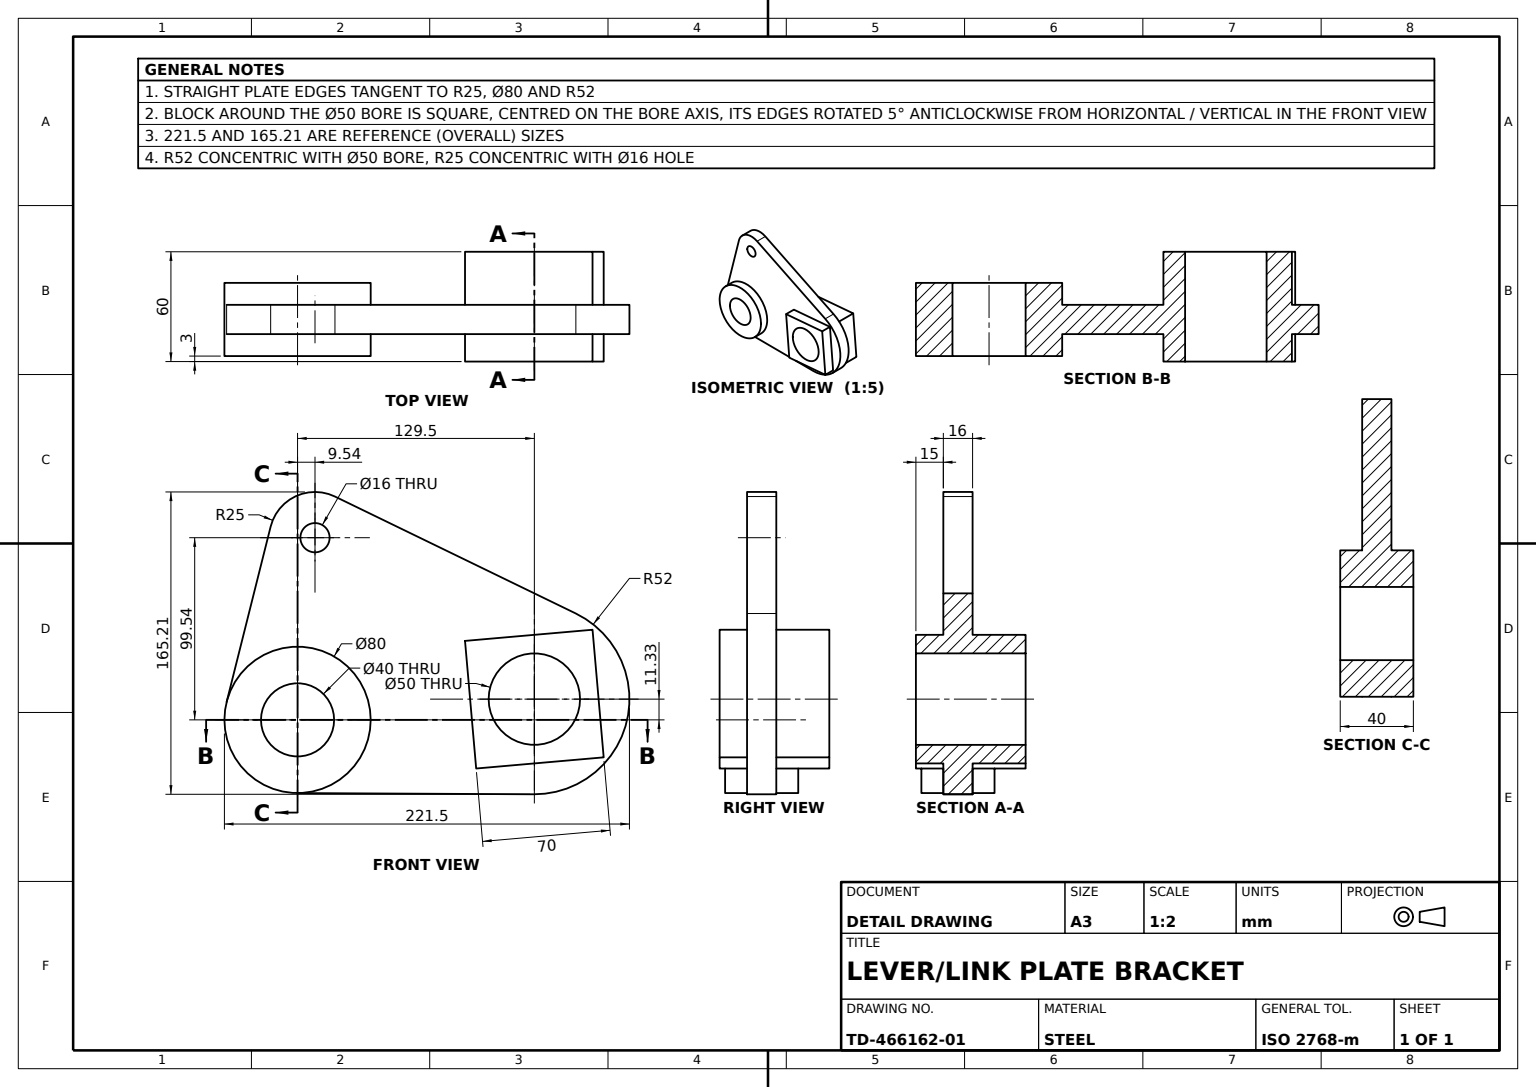
from build123d import *

# Parameters (mm, degrees)
BASE_BLOCK_SKETCH_R              = 40
BASE_BLOCK_SKETCH_R_2            = 20
BASE_BLOCK_40MM_DEPTH            = 20
BRACKET_PLATE_PROFILE_SKETCH_R   = 20
BRACKET_PLATE_PROFILE_SKETCH_R_2 = 8
BRACKET_PLATE_16MM_DEPTH         = 8
BORE_BOSSES_DEPTH                = 15
BORE_BOSSES_DEPTH_BACK           = 45
BORE_BOSSES_START                = 8
SKETCH2_3_R                      = 25


with BuildPart() as part:
    # Base Block Sketch → Base Block 40mm (new, symmetric)
    with BuildSketch(Plane.XY):
        Circle(BASE_BLOCK_SKETCH_R)
        Circle(BASE_BLOCK_SKETCH_R_2, mode=Mode.SUBTRACT)
    extrude(amount=BASE_BLOCK_40MM_DEPTH, both=True)

    # Bracket Plate Profile Sketch → Bracket Plate 16mm (add, symmetric)
    with BuildSketch(Plane.XY):
        with BuildLine():
            ThreePointArc((-38.79460493, 9.74569794), (-31.60581958, -24.516773211), (-0.207064055, -39.999464052))
            Line((-0.207064055, -39.999464052), (129.230816729, -40.669521341))
            ThreePointArc((129.230816729, -40.669521341), (180.148903337, -0.446830099), (152.19937164, 58.1137378))
            Line((152.19937164, 58.1137378), (20.453770296, 122.036129806))
            ThreePointArc((20.453770296, 122.036129806), (-1.027993314, 122.200069977), (-14.706017228, 105.634904541))
            Line((-14.706017228, 105.634904541), (-38.79460493, 9.74569794))
        make_face()
        Circle(BRACKET_PLATE_PROFILE_SKETCH_R, mode=Mode.SUBTRACT)
        Polygon((132.550450996, -23.537032507), (97.683636563, -26.587483503), (94.633185567, 8.27933093), (91.582734571, 43.146145364), (126.449549004, 46.19659636), (161.316363437, 49.247047356), (164.366814433, 14.380232923), (167.417265429, -20.48658151), align=None, mode=Mode.SUBTRACT)
        with Locations((9.540610853, 99.543843328)):
            Circle(BRACKET_PLATE_PROFILE_SKETCH_R_2, mode=Mode.SUBTRACT)
    extrude(amount=BRACKET_PLATE_16MM_DEPTH, both=True)

    # Sketch2_3 → Bore Bosses (add, two sides: drawn at the far end of the back side and taken through both)
    with BuildSketch(Plane.XY.offset(BORE_BOSSES_START - BORE_BOSSES_DEPTH_BACK)):
        Polygon((94.633185567, 8.27933093), (91.582734571, 43.146145364), (126.449549004, 46.19659636), (161.316363437, 49.247047356), (164.366814433, 14.380232923), (167.417265429, -20.48658151), (132.550450996, -23.537032507), (97.683636563, -26.587483503), align=None)
        with Locations((129.5, 11.329781927)):
            Circle(SKETCH2_3_R, mode=Mode.SUBTRACT)
    extrude(amount=BORE_BOSSES_DEPTH + BORE_BOSSES_DEPTH_BACK)


solid = part.part
